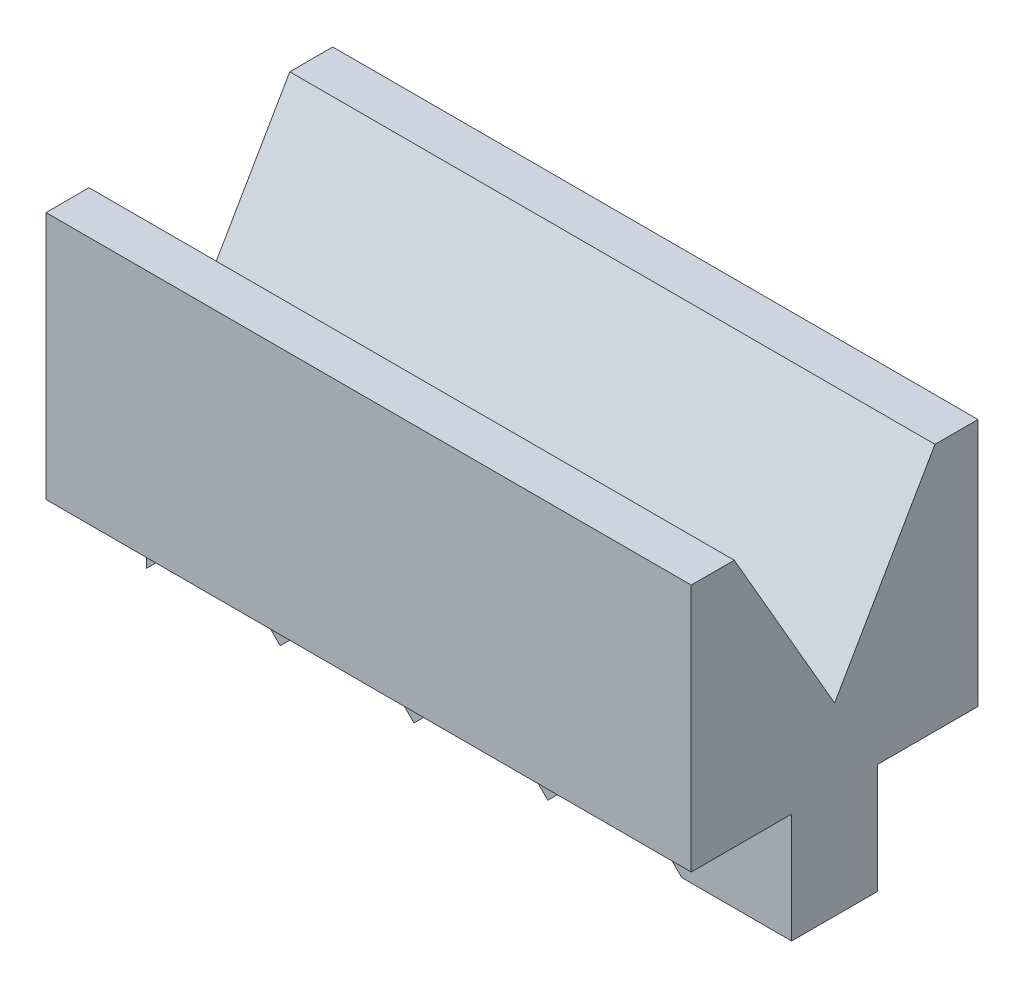
ISO-10303-21;
HEADER;
FILE_DESCRIPTION(('STEP AP214'),'2;1');
FILE_NAME('part.step','',(''),(''),'','','');
FILE_SCHEMA(('AUTOMOTIVE_DESIGN { 1 0 10303 214 1 1 1 1 }'));
ENDSEC;
DATA;
#1=APPLICATION_CONTEXT('core data for automotive mechanical design processes');
#2=APPLICATION_PROTOCOL_DEFINITION('international standard','automotive_design',2000,#1);
#3=PRODUCT_CONTEXT('',#1,'mechanical');
#4=PRODUCT('Part','Part','',(#3));
#5=PRODUCT_RELATED_PRODUCT_CATEGORY('part','',(#4));
#6=PRODUCT_DEFINITION_FORMATION('','',#4);
#7=PRODUCT_DEFINITION_CONTEXT('part definition',#1,'design');
#8=PRODUCT_DEFINITION('design','',#6,#7);
#9=PRODUCT_DEFINITION_SHAPE('','',#8);
#10=(LENGTH_UNIT() NAMED_UNIT(*) SI_UNIT(.MILLI.,.METRE.));
#11=(NAMED_UNIT(*) PLANE_ANGLE_UNIT() SI_UNIT($,.RADIAN.));
#12=(NAMED_UNIT(*) SI_UNIT($,.STERADIAN.) SOLID_ANGLE_UNIT());
#13=UNCERTAINTY_MEASURE_WITH_UNIT(LENGTH_MEASURE(1.E-05),#10,'distance_accuracy_value','');
#14=(GEOMETRIC_REPRESENTATION_CONTEXT(3) GLOBAL_UNCERTAINTY_ASSIGNED_CONTEXT((#13)) GLOBAL_UNIT_ASSIGNED_CONTEXT((#10,
#11,#12)) REPRESENTATION_CONTEXT('',''));
#15=CARTESIAN_POINT('',(0.,0.,0.));
#16=DIRECTION('',(0.,0.,1.));
#17=DIRECTION('',(1.,0.,0.));
#18=AXIS2_PLACEMENT_3D('',#15,#16,#17);
#19=CARTESIAN_POINT('',(-135.,52.,30.));
#20=DIRECTION('',(0.,1.,0.));
#21=DIRECTION('',(0.,0.,1.));
#22=AXIS2_PLACEMENT_3D('',#19,#20,#21);
#23=PLANE('',#22);
#24=DIRECTION('',(0.,0.,1.));
#25=VECTOR('',#24,1.);
#26=CARTESIAN_POINT('',(0.,52.,30.));
#27=LINE('',#26,#25);
#28=CARTESIAN_POINT('',(0.,52.,21.));
#29=VERTEX_POINT('',#28);
#30=CARTESIAN_POINT('',(0.,52.,30.));
#31=VERTEX_POINT('',#30);
#32=EDGE_CURVE('E152',#29,#31,#27,.T.);
#33=ORIENTED_EDGE('',*,*,#32,.F.);
#34=DIRECTION('',(1.,0.,0.));
#35=VECTOR('',#34,1.);
#36=CARTESIAN_POINT('',(-135.,52.,21.));
#37=LINE('',#36,#35);
#38=CARTESIAN_POINT('',(-135.,52.,21.));
#39=VERTEX_POINT('',#38);
#40=EDGE_CURVE('E11',#39,#29,#37,.T.);
#41=ORIENTED_EDGE('',*,*,#40,.F.);
#42=DIRECTION('',(0.,0.,1.));
#43=VECTOR('',#42,1.);
#44=CARTESIAN_POINT('',(-135.,52.,30.));
#45=LINE('',#44,#43);
#46=CARTESIAN_POINT('',(-135.,52.,30.));
#47=VERTEX_POINT('',#46);
#48=EDGE_CURVE('E184',#39,#47,#45,.T.);
#49=ORIENTED_EDGE('',*,*,#48,.T.);
#50=DIRECTION('',(1.,0.,0.));
#51=VECTOR('',#50,1.);
#52=CARTESIAN_POINT('',(-135.,52.,30.));
#53=LINE('',#52,#51);
#54=EDGE_CURVE('E45',#47,#31,#53,.T.);
#55=ORIENTED_EDGE('',*,*,#54,.T.);
#56=EDGE_LOOP('',(#33,#41,#49,#55));
#57=FACE_BOUND('',#56,.T.);
#58=ADVANCED_FACE('F39',(#57),#23,.T.);
#59=CARTESIAN_POINT('',(-135.,52.,21.));
#60=DIRECTION('',(0.,0.500000000000001,-0.866025403784438));
#61=DIRECTION('',(0.,0.866025403784438,0.500000000000001));
#62=AXIS2_PLACEMENT_3D('',#59,#60,#61);
#63=PLANE('',#62);
#64=DIRECTION('',(0.,0.866025403784438,0.500000000000001));
#65=VECTOR('',#64,1.);
#66=CARTESIAN_POINT('',(0.,52.,21.));
#67=LINE('',#66,#65);
#68=CARTESIAN_POINT('',(0.,15.6269330410537,0.));
#69=VERTEX_POINT('',#68);
#70=EDGE_CURVE('E185',#69,#29,#67,.T.);
#71=ORIENTED_EDGE('',*,*,#70,.F.);
#72=DIRECTION('',(1.,0.,0.));
#73=VECTOR('',#72,1.);
#74=CARTESIAN_POINT('',(-135.,15.6269330410537,0.));
#75=LINE('',#74,#73);
#76=CARTESIAN_POINT('',(-135.,15.6269330410537,0.));
#77=VERTEX_POINT('',#76);
#78=EDGE_CURVE('E48',#77,#69,#75,.T.);
#79=ORIENTED_EDGE('',*,*,#78,.F.);
#80=DIRECTION('',(0.,0.866025403784438,0.500000000000001));
#81=VECTOR('',#80,1.);
#82=CARTESIAN_POINT('',(-135.,52.,21.));
#83=LINE('',#82,#81);
#84=EDGE_CURVE('E145',#77,#39,#83,.T.);
#85=ORIENTED_EDGE('',*,*,#84,.T.);
#86=ORIENTED_EDGE('',*,*,#40,.T.);
#87=EDGE_LOOP('',(#71,#79,#85,#86));
#88=FACE_BOUND('',#87,.T.);
#89=ADVANCED_FACE('F205',(#88),#63,.T.);
#90=CARTESIAN_POINT('',(-135.,15.6269330410537,0.));
#91=DIRECTION('',(0.,0.500000000000001,0.866025403784438));
#92=DIRECTION('',(0.,-0.866025403784438,0.500000000000001));
#93=AXIS2_PLACEMENT_3D('',#90,#91,#92);
#94=PLANE('',#93);
#95=DIRECTION('',(0.,-0.866025403784438,0.500000000000001));
#96=VECTOR('',#95,1.);
#97=CARTESIAN_POINT('',(0.,15.6269330410537,0.));
#98=LINE('',#97,#96);
#99=CARTESIAN_POINT('',(0.,52.,-21.));
#100=VERTEX_POINT('',#99);
#101=EDGE_CURVE('E134',#100,#69,#98,.T.);
#102=ORIENTED_EDGE('',*,*,#101,.F.);
#103=DIRECTION('',(1.,0.,0.));
#104=VECTOR('',#103,1.);
#105=CARTESIAN_POINT('',(-135.,52.,-21.));
#106=LINE('',#105,#104);
#107=CARTESIAN_POINT('',(-135.,52.,-21.));
#108=VERTEX_POINT('',#107);
#109=EDGE_CURVE('E127',#108,#100,#106,.T.);
#110=ORIENTED_EDGE('',*,*,#109,.F.);
#111=DIRECTION('',(0.,-0.866025403784438,0.500000000000001));
#112=VECTOR('',#111,1.);
#113=CARTESIAN_POINT('',(-135.,15.6269330410537,0.));
#114=LINE('',#113,#112);
#115=EDGE_CURVE('E129',#108,#77,#114,.T.);
#116=ORIENTED_EDGE('',*,*,#115,.T.);
#117=ORIENTED_EDGE('',*,*,#78,.T.);
#118=EDGE_LOOP('',(#102,#110,#116,#117));
#119=FACE_BOUND('',#118,.T.);
#120=ADVANCED_FACE('F126',(#119),#94,.T.);
#121=CARTESIAN_POINT('',(-135.,52.,-21.));
#122=DIRECTION('',(0.,1.,0.));
#123=DIRECTION('',(0.,0.,1.));
#124=AXIS2_PLACEMENT_3D('',#121,#122,#123);
#125=PLANE('',#124);
#126=DIRECTION('',(0.,0.,1.));
#127=VECTOR('',#126,1.);
#128=CARTESIAN_POINT('',(0.,52.,-21.));
#129=LINE('',#128,#127);
#130=CARTESIAN_POINT('',(0.,52.,-30.));
#131=VERTEX_POINT('',#130);
#132=EDGE_CURVE('E176',#131,#100,#129,.T.);
#133=ORIENTED_EDGE('',*,*,#132,.F.);
#134=DIRECTION('',(1.,0.,0.));
#135=VECTOR('',#134,1.);
#136=CARTESIAN_POINT('',(-135.,52.,-30.));
#137=LINE('',#136,#135);
#138=CARTESIAN_POINT('',(-135.,52.,-30.));
#139=VERTEX_POINT('',#138);
#140=EDGE_CURVE('E137',#139,#131,#137,.T.);
#141=ORIENTED_EDGE('',*,*,#140,.F.);
#142=DIRECTION('',(0.,0.,1.));
#143=VECTOR('',#142,1.);
#144=CARTESIAN_POINT('',(-135.,52.,-21.));
#145=LINE('',#144,#143);
#146=EDGE_CURVE('E142',#139,#108,#145,.T.);
#147=ORIENTED_EDGE('',*,*,#146,.T.);
#148=ORIENTED_EDGE('',*,*,#109,.T.);
#149=EDGE_LOOP('',(#133,#141,#147,#148));
#150=FACE_BOUND('',#149,.T.);
#151=ADVANCED_FACE('F148',(#150),#125,.T.);
#152=CARTESIAN_POINT('',(-135.,0.,-30.));
#153=DIRECTION('',(0.,0.,-1.));
#154=DIRECTION('',(-1.,0.,0.));
#155=AXIS2_PLACEMENT_3D('',#152,#153,#154);
#156=PLANE('',#155);
#157=DIRECTION('',(0.,1.,0.));
#158=VECTOR('',#157,1.);
#159=CARTESIAN_POINT('',(0.,0.,-30.));
#160=LINE('',#159,#158);
#161=CARTESIAN_POINT('',(0.,0.,-30.));
#162=VERTEX_POINT('',#161);
#163=EDGE_CURVE('E177',#162,#131,#160,.T.);
#164=ORIENTED_EDGE('',*,*,#163,.F.);
#165=DIRECTION('',(1.,0.,0.));
#166=VECTOR('',#165,1.);
#167=CARTESIAN_POINT('',(-135.,0.,-30.));
#168=LINE('',#167,#166);
#169=CARTESIAN_POINT('',(-135.,0.,-30.));
#170=VERTEX_POINT('',#169);
#171=EDGE_CURVE('E190',#170,#162,#168,.T.);
#172=ORIENTED_EDGE('',*,*,#171,.F.);
#173=DIRECTION('',(0.,1.,0.));
#174=VECTOR('',#173,1.);
#175=CARTESIAN_POINT('',(-135.,0.,-30.));
#176=LINE('',#175,#174);
#177=EDGE_CURVE('E150',#170,#139,#176,.T.);
#178=ORIENTED_EDGE('',*,*,#177,.T.);
#179=ORIENTED_EDGE('',*,*,#140,.T.);
#180=EDGE_LOOP('',(#164,#172,#178,#179));
#181=FACE_BOUND('',#180,.T.);
#182=ADVANCED_FACE('F214',(#181),#156,.T.);
#183=CARTESIAN_POINT('',(-135.,0.,-9.));
#184=DIRECTION('',(0.,-1.,0.));
#185=DIRECTION('',(0.,0.,-1.));
#186=AXIS2_PLACEMENT_3D('',#183,#184,#185);
#187=PLANE('',#186);
#188=DIRECTION('',(0.,0.,-1.));
#189=VECTOR('',#188,1.);
#190=CARTESIAN_POINT('',(0.,0.,-9.));
#191=LINE('',#190,#189);
#192=CARTESIAN_POINT('',(0.,0.,-9.));
#193=VERTEX_POINT('',#192);
#194=EDGE_CURVE('E175',#193,#162,#191,.T.);
#195=ORIENTED_EDGE('',*,*,#194,.F.);
#196=DIRECTION('',(1.,0.,0.));
#197=VECTOR('',#196,1.);
#198=CARTESIAN_POINT('',(-135.,0.,-9.));
#199=LINE('',#198,#197);
#200=CARTESIAN_POINT('',(-135.,0.,-9.));
#201=VERTEX_POINT('',#200);
#202=EDGE_CURVE('E187',#201,#193,#199,.T.);
#203=ORIENTED_EDGE('',*,*,#202,.F.);
#204=DIRECTION('',(0.,0.,-1.));
#205=VECTOR('',#204,1.);
#206=CARTESIAN_POINT('',(-135.,0.,-9.));
#207=LINE('',#206,#205);
#208=EDGE_CURVE('E149',#201,#170,#207,.T.);
#209=ORIENTED_EDGE('',*,*,#208,.T.);
#210=ORIENTED_EDGE('',*,*,#171,.T.);
#211=EDGE_LOOP('',(#195,#203,#209,#210));
#212=FACE_BOUND('',#211,.T.);
#213=ADVANCED_FACE('F217',(#212),#187,.T.);
#214=CARTESIAN_POINT('',(-135.,-23.,-9.));
#215=DIRECTION('',(0.,0.,-1.));
#216=DIRECTION('',(-1.,0.,0.));
#217=AXIS2_PLACEMENT_3D('',#214,#215,#216);
#218=PLANE('',#217);
#219=DIRECTION('',(0.707106781186544,0.707106781186551,0.));
#220=VECTOR('',#219,1.);
#221=CARTESIAN_POINT('',(-135.,-23.,-9.));
#222=LINE('',#221,#220);
#223=CARTESIAN_POINT('',(-135.,-23.,-9.00000000000001));
#224=VERTEX_POINT('',#223);
#225=CARTESIAN_POINT('',(-121.,-8.99999999999994,-9.00000000000001));
#226=VERTEX_POINT('',#225);
#227=EDGE_CURVE('E283',#224,#226,#222,.T.);
#228=ORIENTED_EDGE('',*,*,#227,.F.);
#229=DIRECTION('',(0.,1.,0.));
#230=VECTOR('',#229,1.);
#231=CARTESIAN_POINT('',(-135.,-23.,-9.));
#232=LINE('',#231,#230);
#233=EDGE_CURVE('E326',#224,#201,#232,.T.);
#234=ORIENTED_EDGE('',*,*,#233,.T.);
#235=ORIENTED_EDGE('',*,*,#202,.T.);
#236=DIRECTION('',(0.,1.,0.));
#237=VECTOR('',#236,1.);
#238=CARTESIAN_POINT('',(0.,-23.,-9.));
#239=LINE('',#238,#237);
#240=CARTESIAN_POINT('',(0.,-23.,-9.));
#241=VERTEX_POINT('',#240);
#242=EDGE_CURVE('E168',#241,#193,#239,.T.);
#243=ORIENTED_EDGE('',*,*,#242,.F.);
#244=DIRECTION('',(1.,0.,0.));
#245=VECTOR('',#244,1.);
#246=CARTESIAN_POINT('',(-135.,-23.,-9.));
#247=LINE('',#246,#245);
#248=CARTESIAN_POINT('',(-22.9999999999999,-23.,-9.));
#249=VERTEX_POINT('',#248);
#250=EDGE_CURVE('E194',#249,#241,#247,.T.);
#251=ORIENTED_EDGE('',*,*,#250,.F.);
#252=DIRECTION('',(0.707106781186548,-0.707106781186547,0.));
#253=VECTOR('',#252,1.);
#254=CARTESIAN_POINT('',(-79.0000000000001,33.0000000000001,-9.));
#255=LINE('',#254,#253);
#256=CARTESIAN_POINT('',(-37.,-8.99999999999995,-9.00000000000001));
#257=VERTEX_POINT('',#256);
#258=EDGE_CURVE('E345',#257,#249,#255,.T.);
#259=ORIENTED_EDGE('',*,*,#258,.F.);
#260=DIRECTION('',(0.707106781186547,0.707106781186548,0.));
#261=VECTOR('',#260,1.);
#262=CARTESIAN_POINT('',(-92.9999999999999,-65.,-9.));
#263=LINE('',#262,#261);
#264=CARTESIAN_POINT('',(-51.,-23.,-9.00000000000001));
#265=VERTEX_POINT('',#264);
#266=EDGE_CURVE('E377',#265,#257,#263,.T.);
#267=ORIENTED_EDGE('',*,*,#266,.F.);
#268=DIRECTION('',(0.707106781186546,-0.707106781186549,0.));
#269=VECTOR('',#268,1.);
#270=CARTESIAN_POINT('',(-92.9999999999998,19.,-9.));
#271=LINE('',#270,#269);
#272=CARTESIAN_POINT('',(-65.,-8.99999999999995,-9.00000000000001));
#273=VERTEX_POINT('',#272);
#274=EDGE_CURVE('E374',#273,#265,#271,.T.);
#275=ORIENTED_EDGE('',*,*,#274,.F.);
#276=DIRECTION('',(0.707106781186547,0.707106781186548,0.));
#277=VECTOR('',#276,1.);
#278=CARTESIAN_POINT('',(-107.,-51.,-9.));
#279=LINE('',#278,#277);
#280=CARTESIAN_POINT('',(-79.,-23.,-9.00000000000001));
#281=VERTEX_POINT('',#280);
#282=EDGE_CURVE('E372',#281,#273,#279,.T.);
#283=ORIENTED_EDGE('',*,*,#282,.F.);
#284=DIRECTION('',(0.707106781186546,-0.707106781186549,0.));
#285=VECTOR('',#284,1.);
#286=CARTESIAN_POINT('',(-107.,5.,-9.));
#287=LINE('',#286,#285);
#288=CARTESIAN_POINT('',(-93.,-8.99999999999995,-9.00000000000001));
#289=VERTEX_POINT('',#288);
#290=EDGE_CURVE('E315',#289,#281,#287,.T.);
#291=ORIENTED_EDGE('',*,*,#290,.F.);
#292=DIRECTION('',(0.707106781186549,0.707106781186546,0.));
#293=VECTOR('',#292,1.);
#294=CARTESIAN_POINT('',(-121.,-37.,-9.));
#295=LINE('',#294,#293);
#296=CARTESIAN_POINT('',(-107.,-22.9999999999999,-9.00000000000001));
#297=VERTEX_POINT('',#296);
#298=EDGE_CURVE('E309',#297,#289,#295,.T.);
#299=ORIENTED_EDGE('',*,*,#298,.F.);
#300=DIRECTION('',(0.707106781186551,-0.707106781186544,0.));
#301=VECTOR('',#300,1.);
#302=CARTESIAN_POINT('',(-121.,-8.99999999999994,-9.));
#303=LINE('',#302,#301);
#304=EDGE_CURVE('E158',#226,#297,#303,.T.);
#305=ORIENTED_EDGE('',*,*,#304,.F.);
#306=EDGE_LOOP('',(#228,#234,#235,#243,#251,#259,#267,#275,#283,#291,#299,#305));
#307=FACE_BOUND('',#306,.T.);
#308=ADVANCED_FACE('F225',(#307),#218,.T.);
#309=CARTESIAN_POINT('',(-135.,-23.,9.));
#310=DIRECTION('',(0.,-1.,0.));
#311=DIRECTION('',(0.,0.,-1.));
#312=AXIS2_PLACEMENT_3D('',#309,#310,#311);
#313=PLANE('',#312);
#314=DIRECTION('',(0.,0.,1.));
#315=VECTOR('',#314,1.);
#316=CARTESIAN_POINT('',(-22.9999999999999,-23.,9.));
#317=LINE('',#316,#315);
#318=CARTESIAN_POINT('',(-22.9999999999999,-23.,9.));
#319=VERTEX_POINT('',#318);
#320=EDGE_CURVE('E296',#249,#319,#317,.T.);
#321=ORIENTED_EDGE('',*,*,#320,.F.);
#322=ORIENTED_EDGE('',*,*,#250,.T.);
#323=DIRECTION('',(0.,0.,-1.));
#324=VECTOR('',#323,1.);
#325=CARTESIAN_POINT('',(0.,-23.,9.));
#326=LINE('',#325,#324);
#327=CARTESIAN_POINT('',(0.,-23.,9.));
#328=VERTEX_POINT('',#327);
#329=EDGE_CURVE('E170',#328,#241,#326,.T.);
#330=ORIENTED_EDGE('',*,*,#329,.F.);
#331=DIRECTION('',(1.,0.,0.));
#332=VECTOR('',#331,1.);
#333=CARTESIAN_POINT('',(-135.,-23.,9.));
#334=LINE('',#333,#332);
#335=EDGE_CURVE('E191',#319,#328,#334,.T.);
#336=ORIENTED_EDGE('',*,*,#335,.F.);
#337=EDGE_LOOP('',(#321,#322,#330,#336));
#338=FACE_BOUND('',#337,.T.);
#339=ADVANCED_FACE('F229',(#338),#313,.T.);
#340=CARTESIAN_POINT('',(-135.,0.,9.));
#341=DIRECTION('',(0.,0.,1.));
#342=DIRECTION('',(0.,-1.,0.));
#343=AXIS2_PLACEMENT_3D('',#340,#341,#342);
#344=PLANE('',#343);
#345=DIRECTION('',(-0.707106781186544,-0.707106781186551,0.));
#346=VECTOR('',#345,1.);
#347=CARTESIAN_POINT('',(-135.,-23.,9.));
#348=LINE('',#347,#346);
#349=CARTESIAN_POINT('',(-121.,-8.99999999999994,9.));
#350=VERTEX_POINT('',#349);
#351=CARTESIAN_POINT('',(-135.,-23.,9.));
#352=VERTEX_POINT('',#351);
#353=EDGE_CURVE('E390',#350,#352,#348,.T.);
#354=ORIENTED_EDGE('',*,*,#353,.F.);
#355=DIRECTION('',(-0.707106781186551,0.707106781186544,0.));
#356=VECTOR('',#355,1.);
#357=CARTESIAN_POINT('',(-121.,-8.99999999999994,9.));
#358=LINE('',#357,#356);
#359=CARTESIAN_POINT('',(-107.,-22.9999999999999,9.));
#360=VERTEX_POINT('',#359);
#361=EDGE_CURVE('E305',#360,#350,#358,.T.);
#362=ORIENTED_EDGE('',*,*,#361,.F.);
#363=DIRECTION('',(-0.707106781186549,-0.707106781186546,0.));
#364=VECTOR('',#363,1.);
#365=CARTESIAN_POINT('',(-93.,-8.99999999999995,9.));
#366=LINE('',#365,#364);
#367=CARTESIAN_POINT('',(-93.,-8.99999999999995,9.));
#368=VERTEX_POINT('',#367);
#369=EDGE_CURVE('E399',#368,#360,#366,.T.);
#370=ORIENTED_EDGE('',*,*,#369,.F.);
#371=DIRECTION('',(-0.707106781186546,0.707106781186549,0.));
#372=VECTOR('',#371,1.);
#373=CARTESIAN_POINT('',(-93.,-8.99999999999995,9.));
#374=LINE('',#373,#372);
#375=CARTESIAN_POINT('',(-79.,-23.,9.));
#376=VERTEX_POINT('',#375);
#377=EDGE_CURVE('E366',#376,#368,#374,.T.);
#378=ORIENTED_EDGE('',*,*,#377,.F.);
#379=DIRECTION('',(-0.707106781186547,-0.707106781186548,0.));
#380=VECTOR('',#379,1.);
#381=CARTESIAN_POINT('',(-79.,-23.,9.));
#382=LINE('',#381,#380);
#383=CARTESIAN_POINT('',(-65.,-8.99999999999995,9.));
#384=VERTEX_POINT('',#383);
#385=EDGE_CURVE('E398',#384,#376,#382,.T.);
#386=ORIENTED_EDGE('',*,*,#385,.F.);
#387=DIRECTION('',(-0.707106781186546,0.707106781186549,0.));
#388=VECTOR('',#387,1.);
#389=CARTESIAN_POINT('',(-65.,-8.99999999999995,9.));
#390=LINE('',#389,#388);
#391=CARTESIAN_POINT('',(-51.,-23.,9.));
#392=VERTEX_POINT('',#391);
#393=EDGE_CURVE('E401',#392,#384,#390,.T.);
#394=ORIENTED_EDGE('',*,*,#393,.F.);
#395=DIRECTION('',(-0.707106781186547,-0.707106781186548,0.));
#396=VECTOR('',#395,1.);
#397=CARTESIAN_POINT('',(-51.,-23.,9.));
#398=LINE('',#397,#396);
#399=CARTESIAN_POINT('',(-37.,-8.99999999999995,9.));
#400=VERTEX_POINT('',#399);
#401=EDGE_CURVE('E409',#400,#392,#398,.T.);
#402=ORIENTED_EDGE('',*,*,#401,.F.);
#403=DIRECTION('',(-0.707106781186548,0.707106781186547,0.));
#404=VECTOR('',#403,1.);
#405=CARTESIAN_POINT('',(-37.,-8.99999999999995,9.));
#406=LINE('',#405,#404);
#407=EDGE_CURVE('E408',#319,#400,#406,.T.);
#408=ORIENTED_EDGE('',*,*,#407,.F.);
#409=ORIENTED_EDGE('',*,*,#335,.T.);
#410=DIRECTION('',(0.,-1.,0.));
#411=VECTOR('',#410,1.);
#412=CARTESIAN_POINT('',(0.,0.,9.));
#413=LINE('',#412,#411);
#414=CARTESIAN_POINT('',(0.,0.,9.));
#415=VERTEX_POINT('',#414);
#416=EDGE_CURVE('E163',#415,#328,#413,.T.);
#417=ORIENTED_EDGE('',*,*,#416,.F.);
#418=DIRECTION('',(1.,0.,0.));
#419=VECTOR('',#418,1.);
#420=CARTESIAN_POINT('',(-135.,0.,9.));
#421=LINE('',#420,#419);
#422=CARTESIAN_POINT('',(-135.,0.,9.));
#423=VERTEX_POINT('',#422);
#424=EDGE_CURVE('E198',#423,#415,#421,.T.);
#425=ORIENTED_EDGE('',*,*,#424,.F.);
#426=DIRECTION('',(0.,-1.,0.));
#427=VECTOR('',#426,1.);
#428=CARTESIAN_POINT('',(-135.,0.,9.));
#429=LINE('',#428,#427);
#430=EDGE_CURVE('E325',#423,#352,#429,.T.);
#431=ORIENTED_EDGE('',*,*,#430,.T.);
#432=EDGE_LOOP('',(#354,#362,#370,#378,#386,#394,#402,#408,#409,#417,#425,#431));
#433=FACE_BOUND('',#432,.T.);
#434=ADVANCED_FACE('F227',(#433),#344,.T.);
#435=CARTESIAN_POINT('',(-135.,0.,30.));
#436=DIRECTION('',(0.,-1.,0.));
#437=DIRECTION('',(0.,0.,-1.));
#438=AXIS2_PLACEMENT_3D('',#435,#436,#437);
#439=PLANE('',#438);
#440=DIRECTION('',(0.,0.,-1.));
#441=VECTOR('',#440,1.);
#442=CARTESIAN_POINT('',(0.,0.,30.));
#443=LINE('',#442,#441);
#444=CARTESIAN_POINT('',(0.,0.,30.));
#445=VERTEX_POINT('',#444);
#446=EDGE_CURVE('E161',#445,#415,#443,.T.);
#447=ORIENTED_EDGE('',*,*,#446,.F.);
#448=DIRECTION('',(1.,0.,0.));
#449=VECTOR('',#448,1.);
#450=CARTESIAN_POINT('',(-135.,0.,30.));
#451=LINE('',#450,#449);
#452=CARTESIAN_POINT('',(-135.,0.,30.));
#453=VERTEX_POINT('',#452);
#454=EDGE_CURVE('E197',#453,#445,#451,.T.);
#455=ORIENTED_EDGE('',*,*,#454,.F.);
#456=DIRECTION('',(0.,0.,-1.));
#457=VECTOR('',#456,1.);
#458=CARTESIAN_POINT('',(-135.,0.,30.));
#459=LINE('',#458,#457);
#460=EDGE_CURVE('E317',#453,#423,#459,.T.);
#461=ORIENTED_EDGE('',*,*,#460,.T.);
#462=ORIENTED_EDGE('',*,*,#424,.T.);
#463=EDGE_LOOP('',(#447,#455,#461,#462));
#464=FACE_BOUND('',#463,.T.);
#465=ADVANCED_FACE('F231',(#464),#439,.T.);
#466=CARTESIAN_POINT('',(-135.,52.,30.));
#467=DIRECTION('',(0.,0.,1.));
#468=DIRECTION('',(0.,-1.,0.));
#469=AXIS2_PLACEMENT_3D('',#466,#467,#468);
#470=PLANE('',#469);
#471=DIRECTION('',(0.,-1.,0.));
#472=VECTOR('',#471,1.);
#473=CARTESIAN_POINT('',(0.,52.,30.));
#474=LINE('',#473,#472);
#475=EDGE_CURVE('E160',#31,#445,#474,.T.);
#476=ORIENTED_EDGE('',*,*,#475,.F.);
#477=ORIENTED_EDGE('',*,*,#54,.F.);
#478=DIRECTION('',(0.,-1.,0.));
#479=VECTOR('',#478,1.);
#480=CARTESIAN_POINT('',(-135.,52.,30.));
#481=LINE('',#480,#479);
#482=EDGE_CURVE('E320',#47,#453,#481,.T.);
#483=ORIENTED_EDGE('',*,*,#482,.T.);
#484=ORIENTED_EDGE('',*,*,#454,.T.);
#485=EDGE_LOOP('',(#476,#477,#483,#484));
#486=FACE_BOUND('',#485,.T.);
#487=ADVANCED_FACE('F200',(#486),#470,.T.);
#488=CARTESIAN_POINT('',(-135.,0.,0.));
#489=DIRECTION('',(1.,0.,0.));
#490=DIRECTION('',(0.,0.,-1.));
#491=AXIS2_PLACEMENT_3D('',#488,#489,#490);
#492=PLANE('',#491);
#493=ORIENTED_EDGE('',*,*,#48,.F.);
#494=ORIENTED_EDGE('',*,*,#84,.F.);
#495=ORIENTED_EDGE('',*,*,#115,.F.);
#496=ORIENTED_EDGE('',*,*,#146,.F.);
#497=ORIENTED_EDGE('',*,*,#177,.F.);
#498=ORIENTED_EDGE('',*,*,#208,.F.);
#499=ORIENTED_EDGE('',*,*,#233,.F.);
#500=DIRECTION('',(0.,0.,-1.));
#501=VECTOR('',#500,1.);
#502=CARTESIAN_POINT('',(-135.,-23.,9.));
#503=LINE('',#502,#501);
#504=EDGE_CURVE('E292',#352,#224,#503,.T.);
#505=ORIENTED_EDGE('',*,*,#504,.F.);
#506=ORIENTED_EDGE('',*,*,#430,.F.);
#507=ORIENTED_EDGE('',*,*,#460,.F.);
#508=ORIENTED_EDGE('',*,*,#482,.F.);
#509=EDGE_LOOP('',(#493,#494,#495,#496,#497,#498,#499,#505,#506,#507,#508));
#510=FACE_BOUND('',#509,.T.);
#511=ADVANCED_FACE('F138',(#510),#492,.F.);
#512=CARTESIAN_POINT('',(0.,0.,0.));
#513=DIRECTION('',(1.,0.,0.));
#514=DIRECTION('',(0.,0.,-1.));
#515=AXIS2_PLACEMENT_3D('',#512,#513,#514);
#516=PLANE('',#515);
#517=ORIENTED_EDGE('',*,*,#32,.T.);
#518=ORIENTED_EDGE('',*,*,#475,.T.);
#519=ORIENTED_EDGE('',*,*,#446,.T.);
#520=ORIENTED_EDGE('',*,*,#416,.T.);
#521=ORIENTED_EDGE('',*,*,#329,.T.);
#522=ORIENTED_EDGE('',*,*,#242,.T.);
#523=ORIENTED_EDGE('',*,*,#194,.T.);
#524=ORIENTED_EDGE('',*,*,#163,.T.);
#525=ORIENTED_EDGE('',*,*,#132,.T.);
#526=ORIENTED_EDGE('',*,*,#101,.T.);
#527=ORIENTED_EDGE('',*,*,#70,.T.);
#528=EDGE_LOOP('',(#517,#518,#519,#520,#521,#522,#523,#524,#525,#526,#527));
#529=FACE_BOUND('',#528,.T.);
#530=ADVANCED_FACE('F203',(#529),#516,.T.);
#531=CARTESIAN_POINT('',(-135.,-23.,-186.));
#532=DIRECTION('',(-0.707106781186551,0.707106781186544,0.));
#533=DIRECTION('',(-0.707106781186544,-0.707106781186551,0.));
#534=AXIS2_PLACEMENT_3D('',#531,#532,#533);
#535=PLANE('',#534);
#536=ORIENTED_EDGE('',*,*,#227,.T.);
#537=DIRECTION('',(0.,0.,1.));
#538=VECTOR('',#537,1.);
#539=CARTESIAN_POINT('',(-121.,-8.99999999999994,-186.));
#540=LINE('',#539,#538);
#541=EDGE_CURVE('E289',#226,#350,#540,.T.);
#542=ORIENTED_EDGE('',*,*,#541,.T.);
#543=ORIENTED_EDGE('',*,*,#353,.T.);
#544=ORIENTED_EDGE('',*,*,#504,.T.);
#545=EDGE_LOOP('',(#536,#542,#543,#544));
#546=FACE_BOUND('',#545,.T.);
#547=ADVANCED_FACE('F247',(#546),#535,.F.);
#548=CARTESIAN_POINT('',(-121.,-8.99999999999994,-186.));
#549=DIRECTION('',(0.707106781186544,0.707106781186551,0.));
#550=DIRECTION('',(-0.707106781186551,0.707106781186544,0.));
#551=AXIS2_PLACEMENT_3D('',#548,#549,#550);
#552=PLANE('',#551);
#553=ORIENTED_EDGE('',*,*,#304,.T.);
#554=DIRECTION('',(0.,0.,1.));
#555=VECTOR('',#554,1.);
#556=CARTESIAN_POINT('',(-107.,-22.9999999999999,-186.));
#557=LINE('',#556,#555);
#558=EDGE_CURVE('E303',#297,#360,#557,.T.);
#559=ORIENTED_EDGE('',*,*,#558,.T.);
#560=ORIENTED_EDGE('',*,*,#361,.T.);
#561=ORIENTED_EDGE('',*,*,#541,.F.);
#562=EDGE_LOOP('',(#553,#559,#560,#561));
#563=FACE_BOUND('',#562,.T.);
#564=ADVANCED_FACE('F271',(#563),#552,.F.);
#565=CARTESIAN_POINT('',(-93.,-8.99999999999995,-186.));
#566=DIRECTION('',(-0.707106781186546,0.707106781186549,0.));
#567=DIRECTION('',(-0.707106781186549,-0.707106781186546,0.));
#568=AXIS2_PLACEMENT_3D('',#565,#566,#567);
#569=PLANE('',#568);
#570=ORIENTED_EDGE('',*,*,#298,.T.);
#571=DIRECTION('',(0.,0.,1.));
#572=VECTOR('',#571,1.);
#573=CARTESIAN_POINT('',(-93.,-8.99999999999995,-186.));
#574=LINE('',#573,#572);
#575=EDGE_CURVE('E361',#289,#368,#574,.T.);
#576=ORIENTED_EDGE('',*,*,#575,.T.);
#577=ORIENTED_EDGE('',*,*,#369,.T.);
#578=ORIENTED_EDGE('',*,*,#558,.F.);
#579=EDGE_LOOP('',(#570,#576,#577,#578));
#580=FACE_BOUND('',#579,.T.);
#581=ADVANCED_FACE('F270',(#580),#569,.F.);
#582=CARTESIAN_POINT('',(-93.,-8.99999999999995,-186.));
#583=DIRECTION('',(0.707106781186549,0.707106781186546,0.));
#584=DIRECTION('',(-0.707106781186546,0.707106781186549,0.));
#585=AXIS2_PLACEMENT_3D('',#582,#583,#584);
#586=PLANE('',#585);
#587=ORIENTED_EDGE('',*,*,#290,.T.);
#588=DIRECTION('',(0.,0.,1.));
#589=VECTOR('',#588,1.);
#590=CARTESIAN_POINT('',(-79.,-23.,-186.));
#591=LINE('',#590,#589);
#592=EDGE_CURVE('E367',#281,#376,#591,.T.);
#593=ORIENTED_EDGE('',*,*,#592,.T.);
#594=ORIENTED_EDGE('',*,*,#377,.T.);
#595=ORIENTED_EDGE('',*,*,#575,.F.);
#596=EDGE_LOOP('',(#587,#593,#594,#595));
#597=FACE_BOUND('',#596,.T.);
#598=ADVANCED_FACE('F263',(#597),#586,.F.);
#599=CARTESIAN_POINT('',(-79.,-23.,-186.));
#600=DIRECTION('',(-0.707106781186548,0.707106781186547,0.));
#601=DIRECTION('',(-0.707106781186547,-0.707106781186548,0.));
#602=AXIS2_PLACEMENT_3D('',#599,#600,#601);
#603=PLANE('',#602);
#604=ORIENTED_EDGE('',*,*,#282,.T.);
#605=DIRECTION('',(0.,0.,1.));
#606=VECTOR('',#605,1.);
#607=CARTESIAN_POINT('',(-65.,-8.99999999999995,-186.));
#608=LINE('',#607,#606);
#609=EDGE_CURVE('E388',#273,#384,#608,.T.);
#610=ORIENTED_EDGE('',*,*,#609,.T.);
#611=ORIENTED_EDGE('',*,*,#385,.T.);
#612=ORIENTED_EDGE('',*,*,#592,.F.);
#613=EDGE_LOOP('',(#604,#610,#611,#612));
#614=FACE_BOUND('',#613,.T.);
#615=ADVANCED_FACE('F259',(#614),#603,.F.);
#616=CARTESIAN_POINT('',(-65.,-8.99999999999995,-186.));
#617=DIRECTION('',(0.707106781186549,0.707106781186546,0.));
#618=DIRECTION('',(-0.707106781186546,0.707106781186549,0.));
#619=AXIS2_PLACEMENT_3D('',#616,#617,#618);
#620=PLANE('',#619);
#621=ORIENTED_EDGE('',*,*,#274,.T.);
#622=DIRECTION('',(0.,0.,1.));
#623=VECTOR('',#622,1.);
#624=CARTESIAN_POINT('',(-51.,-23.,-186.));
#625=LINE('',#624,#623);
#626=EDGE_CURVE('E387',#265,#392,#625,.T.);
#627=ORIENTED_EDGE('',*,*,#626,.T.);
#628=ORIENTED_EDGE('',*,*,#393,.T.);
#629=ORIENTED_EDGE('',*,*,#609,.F.);
#630=EDGE_LOOP('',(#621,#627,#628,#629));
#631=FACE_BOUND('',#630,.T.);
#632=ADVANCED_FACE('F254',(#631),#620,.F.);
#633=CARTESIAN_POINT('',(-51.,-23.,-186.));
#634=DIRECTION('',(-0.707106781186548,0.707106781186547,0.));
#635=DIRECTION('',(-0.707106781186547,-0.707106781186548,0.));
#636=AXIS2_PLACEMENT_3D('',#633,#634,#635);
#637=PLANE('',#636);
#638=ORIENTED_EDGE('',*,*,#266,.T.);
#639=DIRECTION('',(0.,0.,1.));
#640=VECTOR('',#639,1.);
#641=CARTESIAN_POINT('',(-37.,-8.99999999999995,-186.));
#642=LINE('',#641,#640);
#643=EDGE_CURVE('E382',#257,#400,#642,.T.);
#644=ORIENTED_EDGE('',*,*,#643,.T.);
#645=ORIENTED_EDGE('',*,*,#401,.T.);
#646=ORIENTED_EDGE('',*,*,#626,.F.);
#647=EDGE_LOOP('',(#638,#644,#645,#646));
#648=FACE_BOUND('',#647,.T.);
#649=ADVANCED_FACE('F253',(#648),#637,.F.);
#650=CARTESIAN_POINT('',(-37.,-8.99999999999995,-186.));
#651=DIRECTION('',(0.707106781186547,0.707106781186548,0.));
#652=DIRECTION('',(-0.707106781186548,0.707106781186547,0.));
#653=AXIS2_PLACEMENT_3D('',#650,#651,#652);
#654=PLANE('',#653);
#655=ORIENTED_EDGE('',*,*,#258,.T.);
#656=ORIENTED_EDGE('',*,*,#320,.T.);
#657=ORIENTED_EDGE('',*,*,#407,.T.);
#658=ORIENTED_EDGE('',*,*,#643,.F.);
#659=EDGE_LOOP('',(#655,#656,#657,#658));
#660=FACE_BOUND('',#659,.T.);
#661=ADVANCED_FACE('F250',(#660),#654,.F.);
#662=CLOSED_SHELL('',(#58,#89,#120,#151,#182,#213,#308,#339,#434,#465,#487,#511,#530,#547,#564,
#581,#598,#615,#632,#649,#661));
#663=MANIFOLD_SOLID_BREP('B2',#662);
#664=ADVANCED_BREP_SHAPE_REPRESENTATION('',(#18,#663),#14);
#665=SHAPE_DEFINITION_REPRESENTATION(#9,#664);
ENDSEC;
END-ISO-10303-21;
